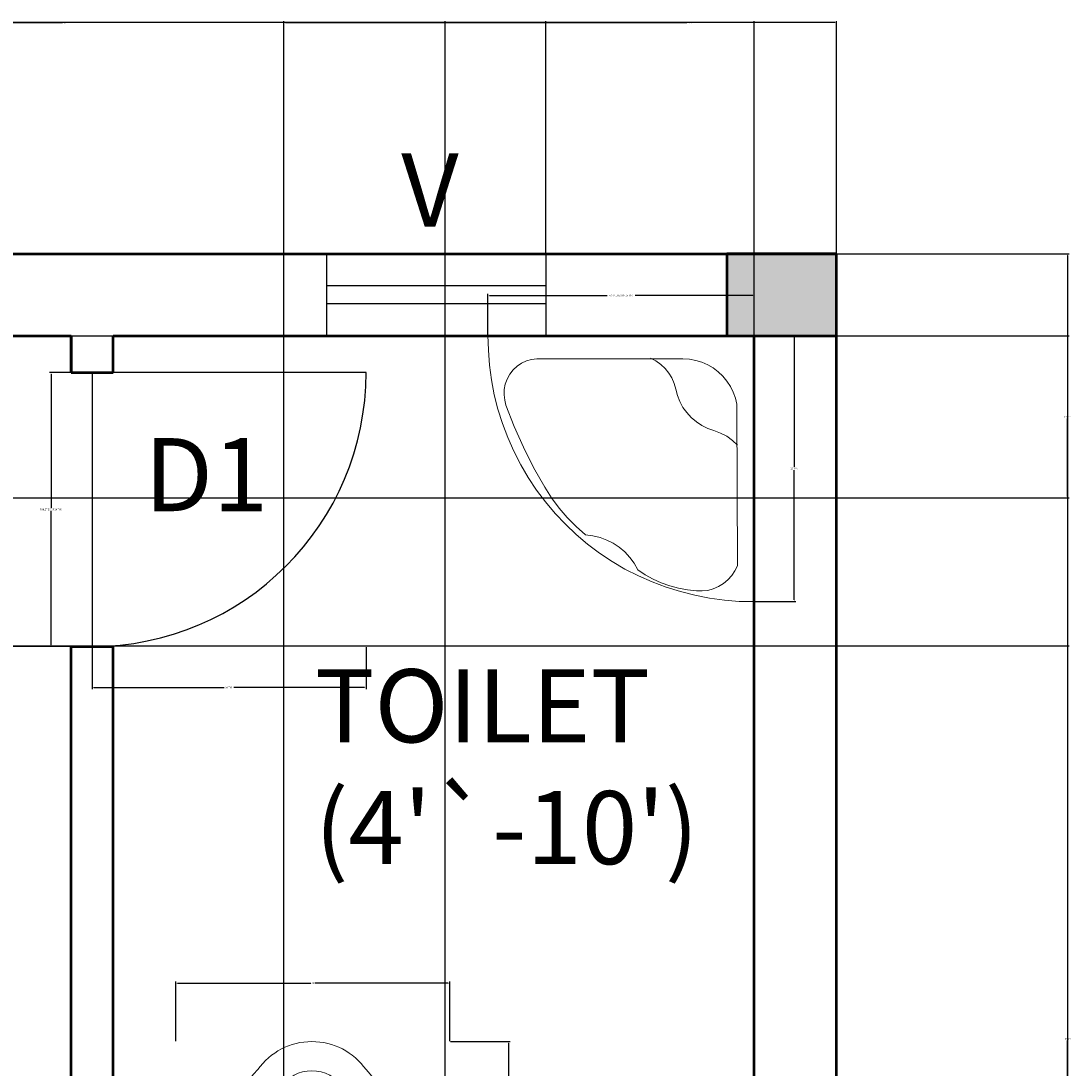
# Model space of a CAD drawing. Units: inches. Extents: x -1517 to -668, y -425 to 52.
# Tile 13 of 13: x -1095 to -980, y -63 to 52. Entities that reach past the tile are written whole.
import ezdxf

# ---------------------------------------------------------------- set-up
doc = ezdxf.new("R2010")
doc.units = ezdxf.units.IN
doc.header["$MEASUREMENT"] = 0
for name, color, linetype, lineweight in [('A-ANNO-DIMS', 2, 'Continuous', 18), ('A-ANNO-TEXT', 7, 'Continuous', 18), ('A-AREA-IDEN', 7, 'Continuous', 25), ('A-COLS-PATT', 252, 'Continuous', 13), ('A-FLOR-FIXT', 9, 'Continuous', 18), ('column', 7, 'Continuous', 50), ('doors', 25, 'Continuous', 25), ('ventilator', 130, 'Continuous', 25), ('walls', 240, 'Continuous', 50)]:
    doc.layers.add(name, color=color, linetype=linetype, lineweight=lineweight)
doc.styles.get("Standard").update_dxf_attribs({"font": 'arial.ttf'})
doc.dimstyles.get("Standard").update_dxf_attribs({"dimtxt": 0.18, "dimasz": 0.18, "dimexe": 0.18, "dimexo": 0.0625, "dimgap": 0.09, "dimtad": 0, "dimtih": 1, "dimtoh": 1, "dimdec": 4, "dimzin": 0, "dimdsep": 46, "dimlunit": 4, "dimtxsty": 'Standard', "dimcen": 0.09, "dimadec": 0, "dimazin": 0, "dimtfac": 1, "dimtdec": 4, "dimtofl": 0, "dimtmove": 0, "dimatfit": 3, "dimfxl": 1, "dimtolj": 1, "dimtzin": 0, "dimarcsym": 0})

# ---------------------------------------------------------------- blocks, each defined once
blk = doc.blocks.new('door 2.6ft')
for p, q in [((0, 30), (0, 0)), ((0, 0), (30, 0))]:
    blk.add_line(p, q)
blk.add_arc((0, 0), 30, 0, 90)
blk = doc.blocks.new('column')
for p, q in [((0, 9), (0, 0)), ((12, 9), (0, 9)), ((12, 0), (12, 9)), ((0, 0), (12, 0))]:
    blk.add_line(p, q)
blk = doc.blocks.new('ventilator 2ft')
for p, q in [((0, 24), (9, 24)), ((3.5, 24), (3.5, 0)), ((5.5, 24), (5.5, 0)), ((0, 0), (9, 0))]:
    blk.add_line(p, q)
blk = doc.blocks.new('A$C1308471B')
at = {"ltscale": 20}
for p, q in [((0.0354, 0.4793), (0.1495, 0.4793)), ((0, 0.4607), (0, 0.0186)), ((0.2013, 0.2397), (0.1923, 0.4384)), ((0.1957, 0.3639), (0.3109, 0.3953)), ((0.4982, 0.3575), (0.4822, 0.3709)), ((0.5021, 0.3528), (0.4724, 0.3528)), ((0.2013, 0.2397), (0.1923, 0.0409)), ((0.5021, 0.1304), (0.4724, 0.1304)), ((0.1959, 0.1193), (0.3109, 0.0879)), ((0.4982, 0.1257), (0.4822, 0.1123)), ((0.0354, 0), (0.1495, 0))]:
    blk.add_line(p, q, dxfattribs=at)
for centre, radius, start, end in [((0.0354, 0.4328), 0.0465, 90, 136.5269), ((0.1495, 0.4365), 0.0429, 2.5755, 90), ((0.006, 0.4607), 0.006, 136.5269, 180), ((0.4248, 0.1104), 0.3068, 47.4135, 111.7924), ((0.4494, 0.2636), 0.1148, 79.3968, 118.5742), ((0.405, 0.2159), 0.153, 63.502, 90.4522), ((0.4658, 0.3513), 0.0255, 50, 79.3968), ((0.3654, 0.2416), 0.1206, 83.3523, 180), ((0.3823, 0.3868), 0.0255, 263.3523, 298.5742), ((0.5146, 0.377), 0.0255, 230, 251.3881), ((0.5021, 0.3273), 0.0255, 70.3751, 90), ((0.4248, 0.1104), 0.2558, 46.612, 70.3751), ((0.5654, 0.2416), 0.116, 0, 54.7115), ((0.5654, 0.2416), 0.065, 0, 57.2974), ((0.3654, 0.2416), 0.1206, 180, 276.6477), ((0.5654, 0.2416), 0.065, 302.7026, 0), ((0.5654, 0.2416), 0.116, 305.2885, 0), ((0.4248, 0.3728), 0.2558, 289.6249, 313.388), ((0.4248, 0.3728), 0.3068, 248.2076, 312.5865), ((0.405, 0.2673), 0.153, 269.5478, 296.498), ((0.5146, 0.1062), 0.0255, 108.6119, 130), ((0.5021, 0.1559), 0.0255, 270, 289.6249), ((0.3823, 0.0964), 0.0255, 61.4258, 96.6477), ((0.4494, 0.2196), 0.1148, 241.4258, 280.6032), ((0.4658, 0.1319), 0.0255, 280.6032, 310), ((0.1495, 0.0429), 0.0429, 270, 357.4245), ((0.006, 0.0186), 0.006, 180, 223.4731), ((0.0354, 0.0465), 0.0465, 223.4731, 270)]:
    blk.add_arc(centre, radius, start, end, dxfattribs=at)
blk = doc.blocks.new('A$C40B42AAA')
for p, q in [((0, 0, -0.3429), (0.0035, 1.4134, -0.3429)), ((0.0035, 1.4134, -0.3429), (1.4134, 1.4134, -0.3429)), ((1.4122, 1.334, -0.3429), (1.4134, 1.4134, -0.3429)), ((0.2714, 1.2869, -0.3429), (0.2427, 1.2685, -0.3429)), ((0.3013, 1.3018, -0.3429), (0.2714, 1.2869, -0.3429)), ((0.3335, 1.3133, -0.3429), (0.3013, 1.3018, -0.3429)), ((0.3335, 1.3133, -0.3429), (0.3657, 1.3214, -0.3429)), ((0.3657, 1.3214, -0.3429), (0.3841, 1.3214, -0.3429)), ((0.3841, 1.3214, -0.3429), (1.2236, 1.3237, -0.3429)), ((0.5578, 1.2972, -0.3429), (0.5359, 1.2673, -0.3429)), ((0.5831, 1.3237, -0.3429), (0.5578, 1.2972, -0.3429)), ((1.2501, 1.311, -0.3429), (1.2236, 1.3237, -0.3429)), ((1.2754, 1.2938, -0.3429), (1.2501, 1.311, -0.3429)), ((1.2972, 1.2731, -0.3429), (1.2754, 1.2938, -0.3429)), ((1.4122, 1.334, -0.3429), (1.4053, 1.2547, -0.3429)), ((0.2162, 1.2466, -0.3429), (0.1932, 1.2225, -0.3429)), ((0.2427, 1.2685, -0.3429), (0.2162, 1.2466, -0.3429)), ((0.5187, 1.234, -0.3429), (0.506, 1.1995, -0.3429)), ((0.5359, 1.2673, -0.3429), (0.5187, 1.234, -0.3429)), ((1.3168, 1.2501, -0.3429), (1.2972, 1.2731, -0.3429)), ((1.3329, 1.2236, -0.3429), (1.3168, 1.2501, -0.3429)), ((1.4053, 1.2547, -0.3429), (1.395, 1.1753, -0.3429)), ((0.1725, 1.1949, -0.3429), (0.1564, 1.1661, -0.3429)), ((0.1932, 1.2225, -0.3429), (0.1725, 1.1949, -0.3429)), ((0.506, 1.1995, -0.3429), (0.4945, 1.1661, -0.3429)), ((1.3455, 1.196, -0.3429), (1.3329, 1.2236, -0.3429)), ((1.3536, 1.1673, -0.3429), (1.3455, 1.196, -0.3429)), ((1.395, 1.1753, -0.3429), (1.38, 1.0983, -0.3429)), ((0.1426, 1.1351, -0.3429), (0.1334, 1.1029, -0.3429)), ((0.1564, 1.1661, -0.3429), (0.1426, 1.1351, -0.3429)), ((0.4784, 1.1351, -0.3429), (0.4589, 1.1063, -0.3429)), ((0.4945, 1.1661, -0.3429), (0.4784, 1.1351, -0.3429)), ((1.357, 1.1374, -0.3429), (1.3536, 1.1673, -0.3429)), ((1.357, 1.1063, -0.3429), (1.357, 1.1374, -0.3429)), ((0.1265, 1.0695, -0.3429), (0.1254, 1.035, -0.3429)), ((0.1334, 1.1029, -0.3429), (0.1265, 1.0695, -0.3429)), ((0.437, 1.0787, -0.3429), (0.4106, 1.0557, -0.3429)), ((0.4589, 1.1063, -0.3429), (0.437, 1.0787, -0.3429)), ((1.3513, 1.0592, -0.3429), (1.3421, 1.012, -0.3429)), ((1.357, 1.1063, -0.3429), (1.3513, 1.0592, -0.3429)), ((1.38, 1.0983, -0.3429), (1.3605, 1.0212, -0.3429)), ((0.1254, 0.2887, -0.3429), (0.1254, 1.035, -0.3429)), ((0.3197, 1.0051, -0.3429), (0.2852, 0.9971, -0.3429)), ((0.3519, 1.0189, -0.3429), (0.3197, 1.0051, -0.3429)), ((0.383, 1.035, -0.3429), (0.3519, 1.0189, -0.3429)), ((0.4106, 1.0557, -0.3429), (0.383, 1.035, -0.3429)), ((1.3421, 1.012, -0.3429), (1.3294, 0.966, -0.3429)), ((1.3605, 1.0212, -0.3429), (1.3375, 0.9453, -0.3429)), ((0.2001, 0.9603, -0.3429), (0.176, 0.9396, -0.3429)), ((0.2266, 0.9764, -0.3429), (0.2001, 0.9603, -0.3429)), ((0.2553, 0.989, -0.3429), (0.2266, 0.9764, -0.3429)), ((0.2852, 0.9971, -0.3429), (0.2553, 0.989, -0.3429)), ((1.3294, 0.966, -0.3429), (1.3133, 0.92, -0.3429)), ((0.1541, 0.9166, -0.3429), (0.1357, 0.8913, -0.3429)), ((0.176, 0.9396, -0.3429), (0.1541, 0.9166, -0.3429)), ((1.3133, 0.92, -0.3429), (1.2938, 0.8763, -0.3429)), ((1.3375, 0.9453, -0.3429), (1.3087, 0.8706, -0.3429)), ((0.1357, 0.8913, -0.3429), (0.1219, 0.8625, -0.3429)), ((1.2938, 0.8763, -0.3429), (1.2708, 0.8349, -0.3429)), ((1.3087, 0.8706, -0.3429), (1.2765, 0.7981, -0.3429)), ((1.2443, 0.7947, -0.3429), (1.2098, 0.7751, -0.3429)), ((1.2765, 0.7981, -0.3429), (1.2409, 0.7268, -0.3429)), ((1.2708, 0.8349, -0.3429), (1.2443, 0.7947, -0.3429)), ((1.15, 0.7268, -0.3429), (1.1247, 0.6969, -0.3429)), ((1.1788, 0.7533, -0.3429), (1.15, 0.7268, -0.3429)), ((1.2098, 0.7751, -0.3429), (1.1788, 0.7533, -0.3429)), ((1.2409, 0.7268, -0.3429), (1.2006, 0.659, -0.3429)), ((1.1247, 0.6969, -0.3429), (1.104, 0.6647, -0.3429)), ((1.0868, 0.6302, -0.3429), (1.073, 0.5946, -0.3429)), ((1.104, 0.6647, -0.3429), (1.0868, 0.6302, -0.3429)), ((1.2006, 0.659, -0.3429), (1.1558, 0.5923, -0.3429)), ((1.073, 0.5946, -0.3429), (1.0638, 0.5566, -0.3429)), ((1.1558, 0.5923, -0.3429), (1.1086, 0.529, -0.3429)), ((1.0592, 0.5175, -0.3429), (1.0155, 0.4681, -0.3429)), ((1.1086, 0.529, -0.3429), (1.0569, 0.4681, -0.3429)), ((1.0638, 0.5566, -0.3429), (1.0592, 0.5175, -0.3429)), ((1.0155, 0.4681, -0.3429), (0.9672, 0.4209, -0.3429)), ((1.0569, 0.4681, -0.3429), (1.0028, 0.4106, -0.3429)), ((0.9672, 0.4209, -0.3429), (0.9166, 0.3772, -0.3429)), ((1.0028, 0.4106, -0.3429), (0.9453, 0.3565, -0.3429)), ((0.8625, 0.337, -0.3429), (0.8062, 0.3013, -0.3429)), ((0.9166, 0.3772, -0.3429), (0.8625, 0.337, -0.3429)), ((0.9453, 0.3565, -0.3429), (0.8844, 0.3048, -0.3429)), ((0.1242, 0.2599, -0.3429), (0.1254, 0.2887, -0.3429)), ((0.8062, 0.3013, -0.3429), (0.7015, 0.2415, -0.3429)), ((0.8844, 0.3048, -0.3429), (0.8211, 0.2576, -0.3429)), ((0.1277, 0.2312, -0.3429), (0.1242, 0.2599, -0.3429)), ((0.1357, 0.2036, -0.3429), (0.1277, 0.2312, -0.3429)), ((0.7015, 0.2415, -0.3429), (0.5934, 0.1886, -0.3429)), ((0.8211, 0.2576, -0.3429), (0.7544, 0.2128, -0.3429)), ((0.1484, 0.1783, -0.3429), (0.1357, 0.2036, -0.3429)), ((0.1645, 0.1541, -0.3429), (0.1484, 0.1783, -0.3429)), ((0.5934, 0.1886, -0.3429), (0.4842, 0.1392, -0.3429)), ((0.6866, 0.1737, -0.3429), (0.6153, 0.1369, -0.3429)), ((0.7544, 0.2128, -0.3429), (0.6866, 0.1737, -0.3429)), ((0.184, 0.1334, -0.3429), (0.1645, 0.1541, -0.3429)), ((0.207, 0.1162, -0.3429), (0.184, 0.1334, -0.3429)), ((0.2323, 0.1012, -0.3429), (0.207, 0.1162, -0.3429)), ((0.4842, 0.1392, -0.3429), (0.3715, 0.0955, -0.3429)), ((0.6153, 0.1369, -0.3429), (0.5428, 0.1047, -0.3429)), ((0.2588, 0.092, -0.3429), (0.2323, 0.1012, -0.3429)), ((0.2875, 0.0863, -0.3429), (0.2588, 0.092, -0.3429)), ((0.3163, 0.0851, -0.3429), (0.2875, 0.0863, -0.3429)), ((0.3439, 0.0886, -0.3429), (0.3163, 0.0851, -0.3429)), ((0.3715, 0.0955, -0.3429), (0.3439, 0.0886, -0.3429)), ((0.3715, 0.0966, -0.3429), (0.3715, 0.0955, -0.3429)), ((0.3715, 0.0955, -0.3429), (0.3715, 0.0966, -0.3429)), ((0.4681, 0.0771, -0.3429), (0.3922, 0.0529, -0.3429)), ((0.5428, 0.1047, -0.3429), (0.4681, 0.0771, -0.3429)), ((0.0794, 0.0023, -0.3429), (0, 0, -0.3429)), ((0.1587, 0.0081, -0.3429), (0.0794, 0.0023, -0.3429)), ((0.2369, 0.0184, -0.3429), (0.1587, 0.0081, -0.3429)), ((0.3151, 0.0334, -0.3429), (0.2369, 0.0184, -0.3429)), ((0.3922, 0.0529, -0.3429), (0.3151, 0.0334, -0.3429))]:
    blk.add_line(p, q)
blk = doc.blocks.new('*D22')
at = {"layer": 'A-ANNO-DIMS', "color": 0, "lineweight": -2, "transparency": 16777216}
for p, q in [((-1087.07, 13.63), (-1091.68, 13.63)), ((-1091.5, 13.45), (-1091.5, -1.19)), ((-1091.5, -16.19), (-1091.5, -1.55)), ((-1087.07, -16.37), (-1091.68, -16.37))]:
    blk.add_line(p, q, dxfattribs=at)
at = {"layer": 'A-ANNO-DIMS', "color": 0, "transparency": 16777216}
for points in [[(-1091.53, 13.45), (-1091.47, 13.45), (-1091.5, 13.63)], [(-1091.53, -16.19), (-1091.47, -16.19), (-1091.5, -16.37)]]:
    blk.add_solid(points, dxfattribs=at)
at = {"layer": 'Defpoints', "color": 0, "transparency": 16777216}
for p in [(-1087, 13.63), (-1091.5, -16.37), (-1087, -16.37)]:
    blk.add_point(p, dxfattribs=at)
at = {"layer": 'A-ANNO-DIMS', "color": 0, "transparency": 16777216, "insert": (-1091.5, -1.37), "char_height": 0.18, "attachment_point": 5}
blk.add_mtext('\\A1;TOILET DOOR 30 TYP.', dxfattribs=at)
blk = doc.blocks.new('*D23')
at = {"layer": 'A-ANNO-DIMS', "color": 0, "lineweight": -2, "transparency": 16777216}
for p, q in [((-1087, -16.43), (-1087, -21.05)), ((-1057, -16.43), (-1057, -21.05)), ((-1086.82, -20.87), (-1072.53, -20.87)), ((-1057.18, -20.87), (-1071.48, -20.87))]:
    blk.add_line(p, q, dxfattribs=at)
at = {"layer": 'A-ANNO-DIMS', "color": 0, "transparency": 16777216}
for points in [[(-1086.82, -20.84), (-1086.82, -20.9), (-1087, -20.87)], [(-1057.18, -20.84), (-1057.18, -20.9), (-1057, -20.87)]]:
    blk.add_solid(points, dxfattribs=at)
at = {"layer": 'Defpoints', "color": 0, "transparency": 16777216}
for p in [(-1087, -16.37), (-1057, -16.37), (-1057, -20.87)]:
    blk.add_point(p, dxfattribs=at)
at = {"layer": 'A-ANNO-DIMS', "color": 0, "transparency": 16777216, "insert": (-1072, -20.87), "char_height": 0.18, "attachment_point": 5}
blk.add_mtext('\\A1;30 TYP.', dxfattribs=at)
blk = doc.blocks.new('*D30')
at = {"layer": 'A-ANNO-DIMS', "color": 0, "lineweight": -2, "transparency": 16777216}
for p, q in [((-1047.75, -59.62), (-1041.24, -59.62)), ((-1041.42, -59.8), (-1041.42, -80.76)), ((-1041.42, -102.09), (-1041.42, -81.13)), ((-1047.75, -102.27), (-1041.24, -102.27))]:
    blk.add_line(p, q, dxfattribs=at)
at = {"layer": 'A-ANNO-DIMS', "color": 0, "transparency": 16777216}
for points in [[(-1041.45, -59.8), (-1041.39, -59.8), (-1041.42, -59.62)], [(-1041.45, -102.09), (-1041.39, -102.09), (-1041.42, -102.27)]]:
    blk.add_solid(points, dxfattribs=at)
at = {"layer": 'Defpoints', "color": 0, "transparency": 16777216}
for p in [(-1047.82, -59.62), (-1041.42, -59.62), (-1047.82, -102.27)]:
    blk.add_point(p, dxfattribs=at)
at = {"layer": 'A-ANNO-DIMS', "color": 0, "transparency": 16777216, "insert": (-1041.42, -80.94), "char_height": 0.18, "attachment_point": 5}
blk.add_mtext('\\A1;WC 43', dxfattribs=at)
blk = doc.blocks.new('*D31')
at = {"layer": 'A-ANNO-DIMS', "color": 0, "lineweight": -2, "transparency": 16777216}
for p, q in [((-1077.82, -59.56), (-1077.82, -53.05)), ((-1077.64, -53.23), (-1063.04, -53.23)), ((-1048, -53.23), (-1062.6, -53.23)), ((-1047.82, -59.56), (-1047.82, -53.05))]:
    blk.add_line(p, q, dxfattribs=at)
at = {"layer": 'A-ANNO-DIMS', "color": 0, "transparency": 16777216}
for points in [[(-1077.64, -53.2), (-1077.64, -53.26), (-1077.82, -53.23)], [(-1048, -53.2), (-1048, -53.26), (-1047.82, -53.23)]]:
    blk.add_solid(points, dxfattribs=at)
at = {"layer": 'Defpoints', "color": 0, "transparency": 16777216}
for p in [(-1077.82, -53.23), (-1077.82, -59.62), (-1047.82, -59.62)]:
    blk.add_point(p, dxfattribs=at)
at = {"layer": 'A-ANNO-DIMS', "color": 0, "transparency": 16777216, "insert": (-1062.82, -53.23), "char_height": 0.18, "attachment_point": 5}
blk.add_mtext('\\A1;30', dxfattribs=at)
blk = doc.blocks.new('*D32')
at = {"layer": 'A-ANNO-DIMS', "color": 0, "lineweight": -2, "transparency": 16777216}
for p, q in [((-1043.66, 17.76), (-1043.66, 22.25)), ((-1043.48, 22.07), (-1030.6, 22.07)), ((-1014.68, 22.07), (-1027.56, 22.07)), ((-1014.5, 17.76), (-1014.5, 22.25))]:
    blk.add_line(p, q, dxfattribs=at)
at = {"layer": 'A-ANNO-DIMS', "color": 0, "transparency": 16777216}
for points in [[(-1043.48, 22.1), (-1043.48, 22.04), (-1043.66, 22.07)], [(-1014.68, 22.1), (-1014.68, 22.04), (-1014.5, 22.07)]]:
    blk.add_solid(points, dxfattribs=at)
at = {"layer": 'Defpoints', "color": 0, "transparency": 16777216}
for p in [(-1014.5, 22.07), (-1043.66, 17.7), (-1014.5, 17.7)]:
    blk.add_point(p, dxfattribs=at)
at = {"layer": 'A-ANNO-DIMS', "color": 0, "transparency": 16777216, "insert": (-1029.08, 22.07), "char_height": 0.18, "attachment_point": 5}
blk.add_mtext('\\A1;CORNER BASIN 29 TYP.', dxfattribs=at)
blk = doc.blocks.new('*D33')
at = {"layer": 'A-ANNO-DIMS', "color": 0, "lineweight": -2, "transparency": 16777216}
for p, q in [((-1014.44, 17.7), (-1009.95, 17.7)), ((-1010.13, 17.52), (-1010.13, 3.31)), ((-1010.13, -11.27), (-1010.13, 2.94)), ((-1014.44, -11.45), (-1009.95, -11.45))]:
    blk.add_line(p, q, dxfattribs=at)
at = {"layer": 'A-ANNO-DIMS', "color": 0, "transparency": 16777216}
for points in [[(-1010.16, 17.52), (-1010.1, 17.52), (-1010.13, 17.7)], [(-1010.16, -11.27), (-1010.1, -11.27), (-1010.13, -11.45)]]:
    blk.add_solid(points, dxfattribs=at)
at = {"layer": 'Defpoints', "color": 0, "transparency": 16777216}
for p in [(-1014.5, 17.7), (-1014.5, -11.45), (-1010.13, -11.45)]:
    blk.add_point(p, dxfattribs=at)
at = {"layer": 'A-ANNO-DIMS', "color": 0, "transparency": 16777216, "insert": (-1010.13, 3.12), "char_height": 0.18, "attachment_point": 5}
blk.add_mtext('\\A1;29 TYP.', dxfattribs=at)
blk = doc.blocks.new('*D46')
at = {"layer": 'A-ANNO-DIMS', "color": 0, "lineweight": -2, "transparency": 16777216}
for p, q in [((-1005.44, 26.63), (-980.02, 26.63)), ((-980.2, 26.45), (-980.2, -127.69)), ((-980.2, -282.19), (-980.2, -128.05)), ((-1005.44, -282.37), (-980.02, -282.37))]:
    blk.add_line(p, q, dxfattribs=at)
at = {"layer": 'A-ANNO-DIMS', "color": 0, "transparency": 16777216}
for points in [[(-980.23, 26.45), (-980.17, 26.45), (-980.2, 26.63)], [(-980.23, -282.19), (-980.17, -282.19), (-980.2, -282.37)]]:
    blk.add_solid(points, dxfattribs=at)
at = {"layer": 'Defpoints', "color": 0, "transparency": 16777216}
for p in [(-1005.5, 26.63), (-1005.5, -282.37), (-980.2, -282.37)]:
    blk.add_point(p, dxfattribs=at)
at = {"layer": 'A-ANNO-DIMS', "color": 0, "transparency": 16777216, "insert": (-980.2, -127.87), "char_height": 0.18, "attachment_point": 5}
blk.add_mtext('\\A1;309', dxfattribs=at)
blk = doc.blocks.new('*D53')
at = {"layer": 'A-ANNO-DIMS', "color": 0, "lineweight": -2, "transparency": 16777216}
for p, q in [((-1242.5, -153.31), (-1242.5, 52.11)), ((-1242.32, 51.93), (-1128.79, 51.93)), ((-1014.68, 51.93), (-1128.21, 51.93)), ((-1014.5, -150.31), (-1014.5, 52.11))]:
    blk.add_line(p, q, dxfattribs=at)
at = {"layer": 'A-ANNO-DIMS', "color": 0, "transparency": 16777216}
for points in [[(-1242.32, 51.96), (-1242.32, 51.9), (-1242.5, 51.93)], [(-1014.68, 51.96), (-1014.68, 51.9), (-1014.5, 51.93)]]:
    blk.add_solid(points, dxfattribs=at)
at = {"layer": 'Defpoints', "color": 0, "transparency": 16777216}
for p in [(-1014.5, 51.93), (-1014.5, -150.37), (-1242.5, -153.37)]:
    blk.add_point(p, dxfattribs=at)
at = {"layer": 'A-ANNO-DIMS', "color": 0, "transparency": 16777216, "insert": (-1128.5, 51.93), "char_height": 0.18, "attachment_point": 5}
blk.add_mtext('\\A1;228', dxfattribs=at)
blk = doc.blocks.new('*D57')
at = {"layer": 'A-ANNO-DIMS', "color": 0, "lineweight": -2, "transparency": 16777216}
for p, q in [((-1114.02, -282.31), (-1114.02, 52.11)), ((-1113.84, 51.93), (-1090.24, 51.93)), ((-1066.2, 51.93), (-1089.8, 51.93)), ((-1066.02, -282.31), (-1066.02, 52.11))]:
    blk.add_line(p, q, dxfattribs=at)
at = {"layer": 'A-ANNO-DIMS', "color": 0, "transparency": 16777216}
for points in [[(-1113.84, 51.96), (-1113.84, 51.9), (-1114.02, 51.93)], [(-1066.2, 51.96), (-1066.2, 51.9), (-1066.02, 51.93)]]:
    blk.add_solid(points, dxfattribs=at)
at = {"layer": 'Defpoints', "color": 0, "transparency": 16777216}
for p in [(-1066.02, 51.93), (-1114.02, -282.37), (-1066.02, -282.37)]:
    blk.add_point(p, dxfattribs=at)
at = {"layer": 'A-ANNO-DIMS', "color": 0, "transparency": 16777216, "insert": (-1090.02, 51.93), "char_height": 0.18, "attachment_point": 5}
blk.add_mtext('\\A1;48', dxfattribs=at)
blk = doc.blocks.new('*D58')
at = {"layer": 'A-ANNO-DIMS', "color": 0, "lineweight": -2, "transparency": 16777216}
for p, q in [((-1066.02, -282.31), (-1066.02, 52.11)), ((-1065.84, 51.93), (-1036.14, 51.93)), ((-1005.68, 51.93), (-1035.38, 51.93)), ((-1005.5, -282.31), (-1005.5, 52.11))]:
    blk.add_line(p, q, dxfattribs=at)
at = {"layer": 'A-ANNO-DIMS', "color": 0, "transparency": 16777216}
for points in [[(-1065.84, 51.96), (-1065.84, 51.9), (-1066.02, 51.93)], [(-1005.68, 51.96), (-1005.68, 51.9), (-1005.5, 51.93)]]:
    blk.add_solid(points, dxfattribs=at)
at = {"layer": 'Defpoints', "color": 0, "transparency": 16777216}
for p in [(-1005.5, 51.93), (-1066.02, -282.37), (-1005.5, -282.37)]:
    blk.add_point(p, dxfattribs=at)
at = {"layer": 'A-ANNO-DIMS', "color": 0, "transparency": 16777216, "insert": (-1035.76, 51.93), "char_height": 0.18, "attachment_point": 5}
blk.add_mtext('\\A1;60.51', dxfattribs=at)
blk = doc.blocks.new('*D62')
at = {"layer": 'A-ANNO-DIMS', "color": 0, "lineweight": -2, "transparency": 16777216}
for p, q in [((-1037.34, 26.69), (-1037.34, 52.11)), ((-1037.16, 51.93), (-1021.88, 51.93)), ((-1005.68, 51.93), (-1020.96, 51.93)), ((-1005.5, 26.69), (-1005.5, 52.11))]:
    blk.add_line(p, q, dxfattribs=at)
at = {"layer": 'A-ANNO-DIMS', "color": 0, "transparency": 16777216}
for points in [[(-1037.16, 51.96), (-1037.16, 51.9), (-1037.34, 51.93)], [(-1005.68, 51.96), (-1005.68, 51.9), (-1005.5, 51.93)]]:
    blk.add_solid(points, dxfattribs=at)
at = {"layer": 'Defpoints', "color": 0, "transparency": 16777216}
for p in [(-1005.5, 51.93), (-1037.34, 26.63), (-1005.5, 26.63)]:
    blk.add_point(p, dxfattribs=at)
at = {"layer": 'A-ANNO-DIMS', "color": 0, "transparency": 16777216, "insert": (-1021.42, 51.93), "char_height": 0.18, "attachment_point": 5}
blk.add_mtext('\\A1;31.836', dxfattribs=at)
blk = doc.blocks.new('*D72')
at = {"layer": 'A-ANNO-DIMS', "color": 0, "lineweight": -2, "transparency": 16777216}
for p, q in [((-1285.84, -16.28), (-980.02, -16.28)), ((-980.2, -16.46), (-980.2, -59.14)), ((-980.2, -102.19), (-980.2, -59.51)), ((-1285.84, -102.37), (-980.02, -102.37))]:
    blk.add_line(p, q, dxfattribs=at)
at = {"layer": 'A-ANNO-DIMS', "color": 0, "transparency": 16777216}
for points in [[(-980.23, -16.46), (-980.17, -16.46), (-980.2, -16.28)], [(-980.23, -102.19), (-980.17, -102.19), (-980.2, -102.37)]]:
    blk.add_solid(points, dxfattribs=at)
at = {"layer": 'Defpoints', "color": 0, "transparency": 16777216}
for p in [(-1285.9, -16.28), (-1285.9, -102.37), (-980.2, -102.37)]:
    blk.add_point(p, dxfattribs=at)
at = {"layer": 'A-ANNO-DIMS', "color": 0, "transparency": 16777216, "insert": (-980.2, -59.33), "char_height": 0.18, "attachment_point": 5}
blk.add_mtext('\\A1;86.09', dxfattribs=at)
blk = doc.blocks.new('*D73')
at = {"layer": 'A-ANNO-DIMS', "color": 0, "lineweight": -2, "transparency": 16777216}
for p, q in [((-1089.37, -16.37), (-1516.98, -16.37)), ((-1516.8, -16.55), (-1516.8, -59.19)), ((-1516.8, -102.19), (-1516.8, -59.55)), ((-1089.37, -102.37), (-1516.98, -102.37))]:
    blk.add_line(p, q, dxfattribs=at)
at = {"layer": 'A-ANNO-DIMS', "color": 0, "transparency": 16777216}
for points in [[(-1516.83, -16.55), (-1516.77, -16.55), (-1516.8, -16.37)], [(-1516.83, -102.19), (-1516.77, -102.19), (-1516.8, -102.37)]]:
    blk.add_solid(points, dxfattribs=at)
at = {"layer": 'Defpoints', "color": 0, "transparency": 16777216}
for p in [(-1089.3, -16.37), (-1516.8, -102.37), (-1089.3, -102.37)]:
    blk.add_point(p, dxfattribs=at)
at = {"layer": 'A-ANNO-DIMS', "color": 0, "transparency": 16777216, "insert": (-1516.8, -59.37), "char_height": 0.18, "attachment_point": 5}
blk.add_mtext('\\A1;86', dxfattribs=at)
blk = doc.blocks.new('*D77')
at = {"layer": 'A-ANNO-DIMS', "color": 0, "lineweight": -2, "transparency": 16777216}
for p, q in [((-1482.44, 17.63), (-980.02, 17.63)), ((-980.2, 17.45), (-980.2, 8.94)), ((-980.2, 0.07), (-980.2, 8.58)), ((-1482.44, -0.11), (-980.02, -0.11))]:
    blk.add_line(p, q, dxfattribs=at)
at = {"layer": 'A-ANNO-DIMS', "color": 0, "transparency": 16777216}
for points in [[(-980.23, 17.45), (-980.17, 17.45), (-980.2, 17.63)], [(-980.23, 0.07), (-980.17, 0.07), (-980.2, -0.11)]]:
    blk.add_solid(points, dxfattribs=at)
at = {"layer": 'Defpoints', "color": 0, "transparency": 16777216}
for p in [(-1482.5, 17.63), (-1482.5, -0.11), (-980.2, -0.11)]:
    blk.add_point(p, dxfattribs=at)
at = {"layer": 'A-ANNO-DIMS', "color": 0, "transparency": 16777216, "insert": (-980.2, 8.76), "char_height": 0.18, "attachment_point": 5}
blk.add_mtext('\\A1;17.744', dxfattribs=at)
blk = doc.blocks.new('*D78')
at = {"layer": 'A-ANNO-DIMS', "color": 0, "lineweight": -2, "transparency": 16777216}
for p, q in [((-1048.34, -101.65), (-1048.34, 52.11)), ((-1048.16, 51.93), (-1031.89, 51.93)), ((-1014.68, 51.93), (-1030.96, 51.93)), ((-1014.5, -102.31), (-1014.5, 52.11))]:
    blk.add_line(p, q, dxfattribs=at)
at = {"layer": 'A-ANNO-DIMS', "color": 0, "transparency": 16777216}
for points in [[(-1048.16, 51.96), (-1048.16, 51.9), (-1048.34, 51.93)], [(-1014.68, 51.96), (-1014.68, 51.9), (-1014.5, 51.93)]]:
    blk.add_solid(points, dxfattribs=at)
at = {"layer": 'Defpoints', "color": 0, "transparency": 16777216}
for p in [(-1048.34, 51.93), (-1048.34, -101.71), (-1014.5, -102.37)]:
    blk.add_point(p, dxfattribs=at)
at = {"layer": 'A-ANNO-DIMS', "color": 0, "transparency": 16777216, "insert": (-1031.42, 51.93), "char_height": 0.18, "attachment_point": 5}
blk.add_mtext('\\A1;33.835', dxfattribs=at)

msp = doc.modelspace()

# ---------------------------------------------------------------- hatches: boundary and pattern name
at = {"layer": 'A-COLS-PATT'}
h = msp.add_hatch(dxfattribs=at)
h.set_pattern_fill('AR-CONC', color=256, scale=0.69)
h.set_pattern_definition([(50, (0, 0), (4.949095, -0.43299), [0.5175, -5.6925]), (355, (0, 0), (-0.957384, 5.190126), [0.414, -4.554]), (100.45144, (0.4124, -0.036), (3.991711, 4.757136), [0.439807, -4.83788]), (46.1842, (0, 1.38), (7.363965, -1.142083), [0.77625, -8.53875]), (96.63564, (0.614, 1.285), (6.449167, 6.72142), [0.65971, -7.256825]), (351.18416, (0, 1.38), (6.449167, 6.72142), [0.621, -6.831]), (21, (0.69, 1.035), (4.118659, -2.77807), [0.5175, -5.6925]), (326, (0.69, 1.035), (1.678876, 5.003535), [0.414, -4.554]), (71.45144, (1.033, 0.8035), (5.797534, 2.225465), [0.439807, -4.83788]), (37.5, (0, 0), (0.083903, 2.2969676), [0, -4.4988, 0, -4.623, 0, -4.57125]), (7.5, (0, 0), (1.81518, 2.721441), [0, -2.6358, 0, -4.3953, 0, -1.74225]), (327.5, (-1.5387, 0), (3.6833748, -0.1556286), [0, -1.725, 0, -5.382, 0, -7.1415]), (317.5, (-2.2287, 0), (4.0239846, 0.6907244), [0, -2.2425, 0, -3.5742, 0, -5.0715])])
h.paths.add_polyline_path([(-1491.5037, 26.63), (-1491.5037, 17.63), (-1479.5037, 17.63), (-1479.5037, 26.63)])
h.paths.add_polyline_path([(-1278.5037, 17.63), (-1278.5037, 26.63), (-1290.5037, 26.63), (-1290.5037, 17.63)])
h.paths.add_polyline_path([(-1177.9037, 26.63), (-1189.9037, 26.63), (-1189.9037, 17.63), (-1177.9037, 17.63)])
h.paths.add_polyline_path([(-1017.5037, 26.63), (-1017.5037, 17.63), (-1005.5037, 17.63), (-1005.5037, 26.63)])
h.paths.add_polyline_path([(-1005.5037, -270.37), (-1014.5037, -270.37), (-1014.5037, -282.37), (-1005.5037, -282.37)])
h.paths.add_polyline_path([(-1247.1037, -282.37), (-1235.1037, -282.37), (-1235.1037, -273.37), (-1247.1037, -273.37)])
h.paths.add_polyline_path([(-1367.1037, -273.37), (-1367.1037, -282.37), (-1355.1037, -282.37), (-1355.1037, -273.37)])
h.paths.add_polyline_path([(-1491.5037, -282.37), (-1479.5037, -282.37), (-1479.5037, -273.37), (-1491.5037, -273.37)])
h.paths.add_polyline_path([(-1482.5037, -145.97), (-1491.5037, -145.97), (-1491.5037, -157.97), (-1482.5037, -157.97)])
h.paths.add_polyline_path([(-1491.5037, -94.97), (-1491.5037, -106.97), (-1482.5037, -106.97), (-1482.5037, -94.97)])

# ---------------------------------------------------------------- linework, layer by layer
at = {"layer": 'walls'}
for p, q in [((-1491.5037, 26.63), (-1005.5037, 26.63)), ((-1005.5037, -282.37), (-1005.5037, 26.63)), ((-1185.3037, 17.63), (-1089.3037, 17.63)), ((-1089.3037, 17.63), (-1089.3037, 13.63)), ((-1089.3037, 13.63), (-1089.3037, 17.63)), ((-1084.7037, 13.63), (-1084.7037, 17.63)), ((-1084.7037, 17.63), (-1014.5037, 17.63)), ((-1014.5037, -102.37), (-1014.5037, 17.63)), ((-1089.3037, 13.63), (-1084.7037, 13.63)), ((-1089.3037, -102.37), (-1089.3037, -16.37)), ((-1089.3037, -16.37), (-1084.7037, -16.37)), ((-1084.7037, -102.37), (-1084.7037, -16.2817))]:
    msp.add_line(p, q, dxfattribs=at)

# ---------------------------------------------------------------- block references
at = {"layer": 'A-FLOR-FIXT'}
for name, p, xscale, yscale, zscale, rotation in [('A$C40B42AAA', (-1043.6581, 17.7012, 7.0724), 20.62789551318069, 20.62789551318069, 20.62789551318069, 270), ('A$C1308471B', (-1047.8167, -102.2668), 62.5850366996167, 62.5850366996167, 62.5850366996167, 89.99999999999999)]:
    msp.add_blockref(name, p, dxfattribs=dict(at, xscale=xscale, yscale=yscale, zscale=zscale, rotation=rotation))
at = {"layer": 'column'}
msp.add_blockref('column', (-1017.5037, 17.63), dxfattribs=at)
at = {"layer": 'doors', "rotation": 270}
msp.add_blockref('door 2.6ft', (-1087.0037, 13.63), dxfattribs=at)
at = {"layer": 'ventilator', "rotation": 270}
msp.add_blockref('ventilator 2ft', (-1061.3392, 26.63), dxfattribs=at)

# ---------------------------------------------------------------- texts
at = {"layer": 'A-ANNO-TEXT', "char_height": 8, "attachment_point": 1}
for s, insert in [('{\\fArial|b1|i0|c0|p34;V}', (-1053.1527, 37.6066)), ('{\\fArial|b1|i0|c0|p34;D1}', (-1081.2789, 6.4431))]:
    msp.add_mtext_dynamic_manual_height_columns(s, width=23.131632, gutter_width=1, heights=[0], dxfattribs=dict(at, insert=insert))
at = {"layer": 'A-AREA-IDEN', "insert": (-1062.6207, -18.8601), "char_height": 8, "attachment_point": 1}
msp.add_mtext_dynamic_manual_height_columns("{\\fArial|b1|i0|c0|p34;TOILET\\P(4'`-10')}", width=39.89549, gutter_width=1, heights=[0], dxfattribs=at)

# ---------------------------------------------------------------- dimensions: what is measured, and where the dimension line sits
at = {"layer": 'A-ANNO-DIMS'}
for base, p1, p2, override, picture, middle in [((-1014.5037, 51.93), (-1242.5037, -153.37), (-1014.5037, -150.37), {"dimdec": 0, "dimlfac": 1, "dimrnd": 0, "dimzin": 0, "dimdsep": 46, "dimlunit": 2}, '*D53', (-1128.5037, 51.93)), ((-1066.0183, 51.93), (-1114.0183, -282.37), (-1066.0183, -282.37), {"dimdec": 0, "dimlfac": 1, "dimrnd": 0, "dimzin": 0, "dimdsep": 46, "dimlunit": 2}, '*D57', (-1090.0183, 51.93)), ((-1005.5037, 51.93), (-1066.0183, -282.37), (-1005.5037, -282.37), {"dimdec": 2, "dimlfac": 1, "dimrnd": 0, "dimzin": 0, "dimdsep": 46, "dimlunit": 2}, '*D58', (-1035.761, 51.93)), ((-1048.3383, 51.93), (-1014.5037, -102.37), (-1048.3383, -101.7142), {"dimdec": 3, "dimlfac": 1, "dimrnd": 0, "dimzin": 0, "dimdsep": 46, "dimlunit": 2}, '*D78', (-1031.421, 51.93)), ((-1005.50368, 51.930012), (-1037.339181, 26.630012), (-1005.50368, 26.630012), {"dimdec": 3, "dimlfac": 1, "dimrnd": 0, "dimzin": 0, "dimdsep": 46, "dimlunit": 2}, '*D62', (-1021.421431, 51.930012))]:
    dim = msp.add_linear_dim(base=base, p1=p1, p2=p2, dimstyle='Standard', override=override, dxfattribs=at)
    dim.commit()
    dim.dimension.update_dxf_attribs({"geometry": picture, "text_midpoint": middle})
for base, p1, p2, angle, override, picture, middle in [((-980.2037, -282.37), (-1005.5037, 26.63), (-1005.5037, -282.37), 90, {"dimdec": 0, "dimlfac": 1, "dimrnd": 0, "dimzin": 0, "dimdsep": 46, "dimlunit": 2}, '*D46', (-980.2037, -127.87)), ((-980.2037, -0.1142), (-1482.5037, 17.63), (-1482.5037, -0.1142), 90, {"dimdec": 3, "dimlfac": 1, "dimrnd": 0, "dimzin": 0, "dimdsep": 46, "dimlunit": 2}, '*D77', (-980.2037, 8.7579)), ((-1516.8037, -102.37), (-1089.3037, -16.37), (-1089.3037, -102.37), 90, {"dimdec": 0, "dimlfac": 1, "dimrnd": 0, "dimzin": 0, "dimdsep": 46, "dimlunit": 2}, '*D73', (-1516.8037, -59.37)), ((-980.2037, -102.37), (-1285.9037, -16.2817), (-1285.9037, -102.37), 90, {"dimdec": 2, "dimlfac": 1, "dimrnd": 0, "dimzin": 0, "dimdsep": 46, "dimlunit": 2}, '*D72', (-980.2037, -59.3258)), ((-1077.8167, -53.2262), (-1047.8167, -59.6228), (-1077.8167, -59.6228), 180, {"dimdec": 0, "dimlfac": 1, "dimrnd": 0, "dimzin": 0, "dimdsep": 46, "dimlunit": 2}, '*D31', (-1062.8167, -53.2262))]:
    dim = msp.add_linear_dim(base=base, p1=p1, p2=p2, angle=angle, dimstyle='Standard', override=override, dxfattribs=at)
    dim.commit()
    dim.dimension.update_dxf_attribs({"geometry": picture, "text_midpoint": middle})
for base, p1, p2, text, picture, middle in [((-1014.5037, 22.0743), (-1043.6581, 17.7012), (-1014.5037, 17.7012), 'CORNER BASIN <> TYP.', '*D32', (-1029.0809, 22.0743)), ((-1057.0037, -20.87), (-1087.0037, -16.37), (-1057.0037, -16.37), '<> TYP.', '*D23', (-1072.0037, -20.87))]:
    dim = msp.add_linear_dim(base=base, p1=p1, p2=p2, text=text, dimstyle='Standard', override={"dimdec": 0, "dimlfac": 1, "dimrnd": 0, "dimzin": 0, "dimdsep": 46, "dimlunit": 2}, dxfattribs=at)
    dim.commit()
    dim.dimension.update_dxf_attribs({"geometry": picture, "text_midpoint": middle})
for base, p1, p2, angle, text, picture, middle in [((-1010.1305, -11.4533), (-1014.5037, 17.7012), (-1014.5037, -11.4533), 270, '<> TYP.', '*D33', (-1010.1305, 3.124)), ((-1091.5037, -16.37), (-1087.0037, 13.63), (-1087.0037, -16.37), 270, 'TOILET DOOR <> TYP.', '*D22', (-1091.5037, -1.37)), ((-1041.4201, -59.6228), (-1047.8167, -102.2668), (-1047.8167, -59.6228), 90, 'WC <>', '*D30', (-1041.4201, -80.9448))]:
    dim = msp.add_linear_dim(base=base, p1=p1, p2=p2, angle=angle, text=text, dimstyle='Standard', override={"dimdec": 0, "dimlfac": 1, "dimrnd": 0, "dimzin": 0, "dimdsep": 46, "dimlunit": 2}, dxfattribs=at)
    dim.commit()
    dim.dimension.update_dxf_attribs({"geometry": picture, "text_midpoint": middle})

doc.saveas('drawing.dxf')
